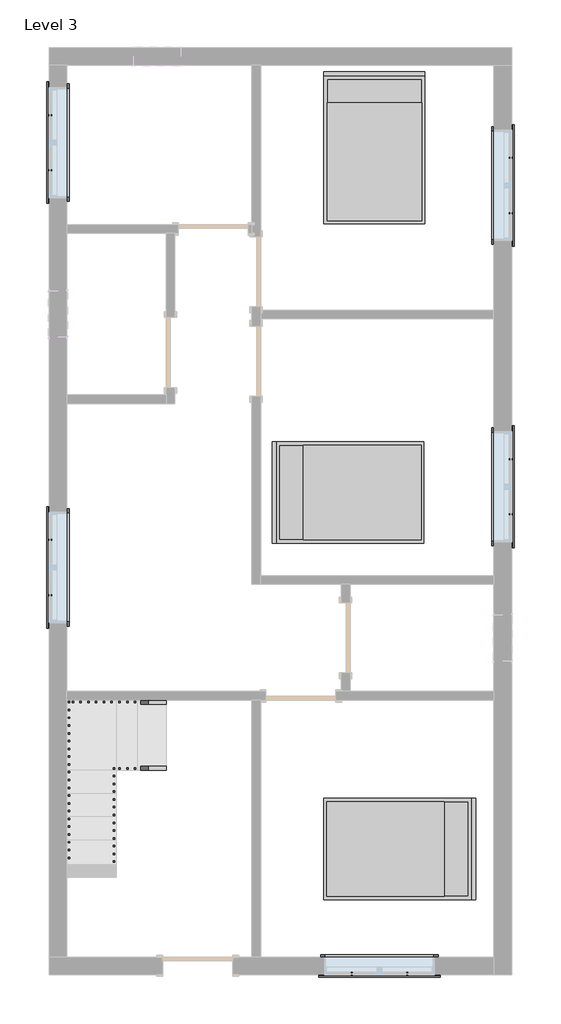
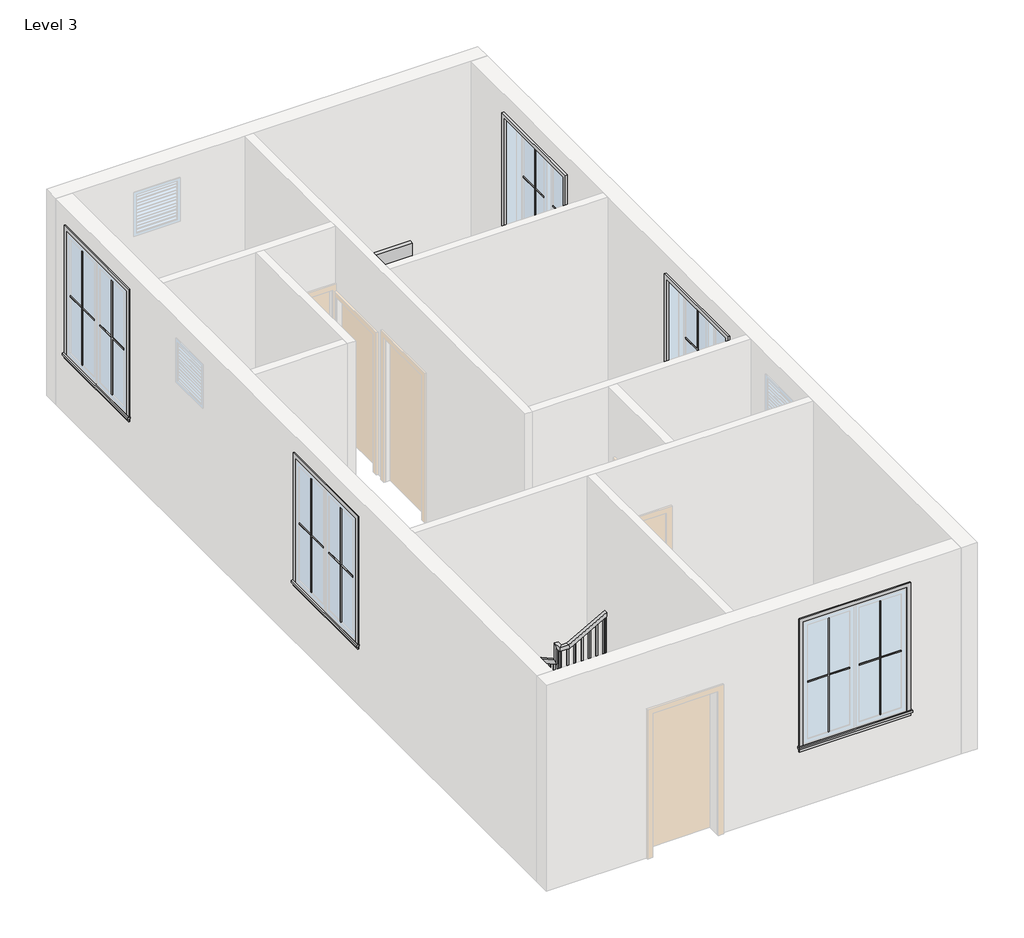
# One storey, part 2 of 2: 20 proxies, 3 furniture elements, 2 railings.
"""IFC4 building model written with IfcOpenShell, lengths in millimetres."""

from ifc_helpers import new_model, si_unit, frame, origin, place, context, project, spatial, polyline, outline, extrude, faceted_brep, transform, mapped, element, save
from components import muntin_pattern_2x2_muntin_pattern_2x2_bff912c5, muntin_pattern_2x2_muntin_pattern_2x2_c2194282, trim_window_exterior_flat_with_sill_e04b3088, trim_window_interior_flat_picture_frame_2a7685fe, bed_17739_bed_17739_15c61121

model = new_model("IFC4")

# Units and contexts
model_context = context("Model", 3, world=origin())
ifc_project = project(units=[si_unit("LENGTHUNIT", "METRE", prefix="MILLI")], contexts=[model_context])

# Site, building, storey
site = spatial("IfcSite", under=ifc_project)
building = spatial("IfcBuilding", under=site)
storey = spatial("IfcBuildingStorey", under=building, Name="Level 3", Elevation=3200.4)

# Proxies
placement = place(None, origin())
muntin_pattern_2x2_muntin_pattern_2x2_shape = muntin_pattern_2x2_muntin_pattern_2x2_bff912c5(model_context)
element("IfcBuildingElementProxy", 1, Name="Muntin Pattern_2x2 : Muntin Pattern_2x2", ObjectType="Muntin Pattern_2x2 : Muntin Pattern_2x2", at=placement, inside=storey, context=model_context, shape_type="MappedRepresentation", body=[
    mapped(muntin_pattern_2x2_muntin_pattern_2x2_shape, transform((-4261.9639285, 4584.2694249, 4184.65), x_axis=(0.0, 1.0, 0.0), y_axis=(-1.0, 0.0, 0.0), z_axis=(0.0, 0.0, 1.0))),
])
element("IfcBuildingElementProxy", 2, Name="Muntin Pattern_2x2 : Muntin Pattern_2x2", ObjectType="Muntin Pattern_2x2 : Muntin Pattern_2x2", at=placement, inside=storey, context=model_context, shape_type="MappedRepresentation", body=[
    mapped(muntin_pattern_2x2_muntin_pattern_2x2_shape, transform((1751.4860715, 4746.1944249, 4184.65), x_axis=(0.0, -1.0, 0.0), y_axis=(1.0, 0.0, 0.0), z_axis=(0.0, 0.0, 1.0))),
])
element("IfcBuildingElementProxy", 3, Name="Muntin Pattern_2x2 : Muntin Pattern_2x2", ObjectType="Muntin Pattern_2x2 : Muntin Pattern_2x2", at=placement, inside=storey, context=model_context, shape_type="MappedRepresentation", body=[
    mapped(muntin_pattern_2x2_muntin_pattern_2x2_shape, transform((-4261.9639285, -962.4555751, 4184.65), x_axis=(0.0, 1.0, 0.0), y_axis=(-1.0, 0.0, 0.0), z_axis=(0.0, 0.0, 1.0))),
])
element("IfcBuildingElementProxy", 4, Name="Muntin Pattern_2x2 : Muntin Pattern_2x2", ObjectType="Muntin Pattern_2x2 : Muntin Pattern_2x2", at=placement, inside=storey, context=model_context, shape_type="MappedRepresentation", body=[
    mapped(muntin_pattern_2x2_muntin_pattern_2x2_shape, transform((1751.4860715, 812.3694249, 4184.65), x_axis=(0.0, -1.0, 0.0), y_axis=(1.0, 0.0, 0.0), z_axis=(0.0, 0.0, 1.0))),
])
element("IfcBuildingElementProxy", 5, Name="Muntin Pattern_2x2 : Muntin Pattern_2x2", ObjectType="Muntin Pattern_2x2 : Muntin Pattern_2x2", at=placement, inside=storey, context=model_context, shape_type="MappedRepresentation", body=[
    mapped(muntin_pattern_2x2_muntin_pattern_2x2_shape, transform((397.3485715, -5907.5180751, 4184.65), x_axis=(-1.0, 0.0, 0.0), y_axis=(0.0, -1.0, 0.0), z_axis=(0.0, 0.0, 1.0))),
])
muntin_pattern_2x2_muntin_pattern_2x2_2_shape = muntin_pattern_2x2_muntin_pattern_2x2_c2194282(model_context)
element("IfcBuildingElementProxy", 6, Name="Muntin Pattern_2x2 : Muntin Pattern_2x2", ObjectType="Muntin Pattern_2x2 : Muntin Pattern_2x2", at=placement, inside=storey, context=model_context, shape_type="MappedRepresentation", body=[
    mapped(muntin_pattern_2x2_muntin_pattern_2x2_2_shape, transform((-4261.9639285, 5304.9944249, 4184.65), x_axis=(0.0, -1.0, 0.0), y_axis=(1.0, 0.0, 0.0), z_axis=(0.0, 0.0, 1.0))),
])
element("IfcBuildingElementProxy", 7, Name="Muntin Pattern_2x2 : Muntin Pattern_2x2", ObjectType="Muntin Pattern_2x2 : Muntin Pattern_2x2", at=placement, inside=storey, context=model_context, shape_type="MappedRepresentation", body=[
    mapped(muntin_pattern_2x2_muntin_pattern_2x2_2_shape, transform((1751.4860715, 4025.4694249, 4184.65), x_axis=(0.0, 1.0, 0.0), y_axis=(-1.0, 0.0, 0.0), z_axis=(0.0, 0.0, 1.0))),
])
element("IfcBuildingElementProxy", 8, Name="Muntin Pattern_2x2 : Muntin Pattern_2x2", ObjectType="Muntin Pattern_2x2 : Muntin Pattern_2x2", at=placement, inside=storey, context=model_context, shape_type="MappedRepresentation", body=[
    mapped(muntin_pattern_2x2_muntin_pattern_2x2_2_shape, transform((-4261.9639285, -241.7305751, 4184.65), x_axis=(0.0, -1.0, 0.0), y_axis=(1.0, 0.0, 0.0), z_axis=(0.0, 0.0, 1.0))),
])
element("IfcBuildingElementProxy", 9, Name="Muntin Pattern_2x2 : Muntin Pattern_2x2", ObjectType="Muntin Pattern_2x2 : Muntin Pattern_2x2", at=placement, inside=storey, context=model_context, shape_type="MappedRepresentation", body=[
    mapped(muntin_pattern_2x2_muntin_pattern_2x2_2_shape, transform((1751.4860715, 91.6444249, 4184.65), x_axis=(0.0, 1.0, 0.0), y_axis=(-1.0, 0.0, 0.0), z_axis=(0.0, 0.0, 1.0))),
])
element("IfcBuildingElementProxy", 10, Name="Muntin Pattern_2x2 : Muntin Pattern_2x2", ObjectType="Muntin Pattern_2x2 : Muntin Pattern_2x2", at=placement, inside=storey, context=model_context, shape_type="MappedRepresentation", body=[
    mapped(muntin_pattern_2x2_muntin_pattern_2x2_2_shape, transform((-323.3764285, -5907.5180751, 4184.65), x_axis=(1.0, 0.0, 0.0), y_axis=(0.0, 1.0, 0.0), z_axis=(0.0, 0.0, 1.0))),
])
trim_window_exterior_flat_with_sill_shape = trim_window_exterior_flat_with_sill_e04b3088(model_context)
element("IfcBuildingElementProxy", 11, Name="Trim-Window-Exterior-Flat : with Sill", ObjectType="Trim-Window-Exterior-Flat : with Sill", at=placement, inside=storey, context=model_context, shape_type="MappedRepresentation", body=[
    mapped(trim_window_exterior_flat_with_sill_shape, transform((-4271.4889285, 4944.6319249, 5943.6), x_axis=(0.0, -1.0, 0.0), y_axis=(0.0, 0.0, 1.0), z_axis=(-1.0, 0.0, 0.0))),
])
element("IfcBuildingElementProxy", 12, Name="Trim-Window-Exterior-Flat : with Sill", ObjectType="Trim-Window-Exterior-Flat : with Sill", at=placement, inside=storey, context=model_context, shape_type="MappedRepresentation", body=[
    mapped(trim_window_exterior_flat_with_sill_shape, transform((1761.0110715, 4385.8319249, 5943.6), x_axis=(0.0, 1.0, 0.0), y_axis=(0.0, 0.0, 1.0), z_axis=(1.0, 0.0, 0.0))),
])
element("IfcBuildingElementProxy", 13, Name="Trim-Window-Exterior-Flat : with Sill", ObjectType="Trim-Window-Exterior-Flat : with Sill", at=placement, inside=storey, context=model_context, shape_type="MappedRepresentation", body=[
    mapped(trim_window_exterior_flat_with_sill_shape, transform((-4271.4889285, -602.0930751, 5943.6), x_axis=(0.0, -1.0, 0.0), y_axis=(0.0, 0.0, 1.0), z_axis=(-1.0, 0.0, 0.0))),
])
element("IfcBuildingElementProxy", 14, Name="Trim-Window-Exterior-Flat : with Sill", ObjectType="Trim-Window-Exterior-Flat : with Sill", at=placement, inside=storey, context=model_context, shape_type="MappedRepresentation", body=[
    mapped(trim_window_exterior_flat_with_sill_shape, transform((1761.0110715, 452.0069249, 5943.6), x_axis=(0.0, 1.0, 0.0), y_axis=(0.0, 0.0, 1.0), z_axis=(1.0, 0.0, 0.0))),
])
element("IfcBuildingElementProxy", 15, Name="Trim-Window-Exterior-Flat : with Sill", ObjectType="Trim-Window-Exterior-Flat : with Sill", at=placement, inside=storey, context=model_context, shape_type="MappedRepresentation", body=[
    mapped(trim_window_exterior_flat_with_sill_shape, transform((36.9860715, -5917.0430751, 5943.6), x_axis=(1.0, 0.0, 0.0), y_axis=(0.0, 0.0, 1.0), z_axis=(0.0, -1.0, 0.0))),
])
trim_window_interior_flat_picture_frame_shape = trim_window_interior_flat_picture_frame_2a7685fe(model_context)
element("IfcBuildingElementProxy", 16, Name="Trim-Window-Interior-Flat : Picture Frame", ObjectType="Trim-Window-Interior-Flat : Picture Frame", at=placement, inside=storey, context=model_context, shape_type="MappedRepresentation", body=[
    mapped(trim_window_interior_flat_picture_frame_shape, transform((-4042.8889285, 4944.6319249, 5943.6), x_axis=(0.0, 1.0, 0.0), y_axis=(0.0, 0.0, 1.0), z_axis=(1.0, 0.0, 0.0))),
])
element("IfcBuildingElementProxy", 17, Name="Trim-Window-Interior-Flat : Picture Frame", ObjectType="Trim-Window-Interior-Flat : Picture Frame", at=placement, inside=storey, context=model_context, shape_type="MappedRepresentation", body=[
    mapped(trim_window_interior_flat_picture_frame_shape, transform((1532.4110715, 4385.8319249, 5943.6), x_axis=(0.0, -1.0, 0.0), y_axis=(0.0, 0.0, 1.0), z_axis=(-1.0, 0.0, 0.0))),
])
element("IfcBuildingElementProxy", 18, Name="Trim-Window-Interior-Flat : Picture Frame", ObjectType="Trim-Window-Interior-Flat : Picture Frame", at=placement, inside=storey, context=model_context, shape_type="MappedRepresentation", body=[
    mapped(trim_window_interior_flat_picture_frame_shape, transform((-4042.8889285, -602.0930751, 5943.6), x_axis=(0.0, 1.0, 0.0), y_axis=(0.0, 0.0, 1.0), z_axis=(1.0, 0.0, 0.0))),
])
element("IfcBuildingElementProxy", 19, Name="Trim-Window-Interior-Flat : Picture Frame", ObjectType="Trim-Window-Interior-Flat : Picture Frame", at=placement, inside=storey, context=model_context, shape_type="MappedRepresentation", body=[
    mapped(trim_window_interior_flat_picture_frame_shape, transform((1532.4110715, 452.0069249, 5943.6), x_axis=(0.0, -1.0, 0.0), y_axis=(0.0, 0.0, 1.0), z_axis=(-1.0, 0.0, 0.0))),
])
element("IfcBuildingElementProxy", 20, Name="Trim-Window-Interior-Flat : Picture Frame", ObjectType="Trim-Window-Interior-Flat : Picture Frame", at=placement, inside=storey, context=model_context, shape_type="MappedRepresentation", body=[
    mapped(trim_window_interior_flat_picture_frame_shape, transform((36.9860715, -5688.4430751, 5943.6), x_axis=(-1.0, 0.0, 0.0), y_axis=(0.0, 0.0, 1.0), z_axis=(0.0, 1.0, 0.0))),
])

# Furniture
bed_17739_bed_17739_shape = bed_17739_bed_17739_15c61121(model_context)
element("IfcFurniture", 21, ObjectType="Bed_17739 : Bed_17739", at=placement, inside=storey, context=model_context, shape_type="MappedRepresentation", body=[
    mapped(bed_17739_bed_17739_shape, transform((-29.6889285, 4852.5569249, 3200.4), x_axis=(1.0, 0.0, 0.0), y_axis=(0.0, 1.0, 0.0), z_axis=(0.0, 0.0, 1.0))),
])
element("IfcFurniture", 22, ObjectType="Bed_17739 : Bed_17739", at=placement, inside=storey, context=model_context, shape_type="MappedRepresentation", body=[
    mapped(bed_17739_bed_17739_shape, transform((-347.1889285, 375.8069249, 3200.4), x_axis=(0.0, 1.0, 0.0), y_axis=(-1.0, 0.0, 0.0), z_axis=(0.0, 0.0, 1.0))),
])
element("IfcFurniture", 23, ObjectType="Bed_17739 : Bed_17739", at=placement, inside=storey, context=model_context, shape_type="MappedRepresentation", body=[
    mapped(bed_17739_bed_17739_shape, transform((275.1110715, -4278.7430751, 3200.4), x_axis=(0.0, -1.0, 0.0), y_axis=(1.0, 0.0, 0.0), z_axis=(0.0, 0.0, 1.0))),
])

# Railings
element("IfcRailing", 24, ObjectType="Handrail - Rectangular", at=placement, inside=storey, context=model_context, shape_type="SolidModel", body=[
    faceted_brep([(-2747.4889285, -2386.4430751, 4284.1333333), (-2747.4889285, -2386.4430751, 4226.9271159), (-2747.4889285, -2335.6430751, 4226.9271159), (-2747.4889285, -2335.6430751, 4284.1333333), (-3396.0267484, -2386.4430751, 4619.9457967), (-3408.3987558, -2386.4430751, 4569.1457967), (-3408.3987558, -2335.6430751, 4569.1457967), (-3396.0267484, -2335.6430751, 4619.9457967), (-3992.0889285, -2386.4430751, 4619.9457967), (-3992.0889285, -2386.4430751, 4569.1457967), (-4042.8889285, -2335.6430751, 4569.1457967), (-4042.8889285, -2335.6430751, 4619.9457967), (-3992.0889285, -2940.1628326, 4619.9457967), (-3992.0889285, -2953.3285634, 4569.1457967), (-4042.8889285, -2953.3285634, 4569.1457967), (-4042.8889285, -2940.1628326, 4619.9457967), (-3992.0889285, -5061.9991591, 5798.9618165), (-3992.0889285, -5075.1648899, 5748.1618165), (-4042.8889285, -5075.1648899, 5748.1618165), (-4042.8889285, -5061.9991591, 5798.9618165), (-3992.0889285, -5637.6430751, 5798.9618165), (-3992.0889285, -5637.6430751, 5748.1618165), (-4042.8889285, -5688.4430751, 5748.1618165), (-4042.8889285, -5688.4430751, 5798.9618165), (-3418.001852, -5637.6430751, 5798.9618165), (-3404.8062484, -5637.6430751, 5748.1618165), (-3404.8062484, -5688.4430751, 5748.1618165), (-3418.001852, -5688.4430751, 5798.9618165), (-2793.6303845, -5637.6430751, 6146.8), (-2793.6303845, -5688.4430751, 6146.8), (-2793.6303845, -5688.4430751, 6088.6487115), (-2793.6303845, -5637.6430751, 6088.6487115)], [[[0, 1, 2, 3]], [[1, 0, 4, 5]], [[2, 1, 5, 6]], [[3, 2, 6, 7]], [[0, 3, 7, 4]], [[5, 4, 8, 9]], [[6, 5, 9, 10]], [[7, 6, 10, 11]], [[4, 7, 11, 8]], [[9, 8, 12, 13]], [[10, 9, 13, 14]], [[11, 10, 14, 15]], [[8, 11, 15, 12]], [[13, 12, 16, 17]], [[14, 13, 17, 18]], [[15, 14, 18, 19]], [[12, 15, 19, 16]], [[17, 16, 20, 21]], [[18, 17, 21, 22]], [[19, 18, 22, 23]], [[16, 19, 23, 20]], [[21, 20, 24, 25]], [[22, 21, 25, 26]], [[23, 22, 26, 27]], [[20, 23, 27, 24]], [[28, 29, 30, 31]], [[25, 24, 28, 31]], [[26, 25, 31, 30]], [[27, 26, 30, 29]], [[24, 27, 29, 28]]]),
    extrude(outline(polyline([(6091.3598207, -2788.7639285), (6080.7470401, -2807.8139285), (5063.0666667, -2807.8139285), (5063.0666667, -2788.7639285), (6091.3598207, -2788.7639285)])), frame((0.0, -5672.5680751, 0.0), z_axis=(0.0, 1.0, 0.0), x_axis=(0.0, 0.0, 1.0)), (0.0, 0.0, 1.0), 19.05),
    extrude(outline(polyline([(6034.7583242, -2890.3639285), (6024.1455436, -2909.4139285), (5063.0666667, -2909.4139285), (5063.0666667, -2890.3639285), (6034.7583242, -2890.3639285)])), frame((0.0, -5672.5680751, 0.0), z_axis=(0.0, 1.0, 0.0), x_axis=(0.0, 0.0, 1.0)), (0.0, 0.0, 1.0), 19.05),
    extrude(outline(polyline([(5978.1568277, -2991.9639285), (5967.5440471, -3011.0139285), (5063.0666667, -3011.0139285), (5063.0666667, -2991.9639285), (5978.1568277, -2991.9639285)])), frame((0.0, -5672.5680751, 0.0), z_axis=(0.0, 1.0, 0.0), x_axis=(0.0, 0.0, 1.0)), (0.0, 0.0, 1.0), 19.05),
    extrude(outline(polyline([(5921.5553312, -3093.5639285), (5910.9425506, -3112.6139285), (5063.0666667, -3112.6139285), (5063.0666667, -3093.5639285), (5921.5553312, -3093.5639285)])), frame((0.0, -5672.5680751, 0.0), z_axis=(0.0, 1.0, 0.0), x_axis=(0.0, 0.0, 1.0)), (0.0, 0.0, 1.0), 19.05),
    extrude(outline(polyline([(5864.9538346, -3195.1639285), (5854.3410541, -3214.2139285), (4893.7333333, -3214.2139285), (4893.7333333, -3195.1639285), (5864.9538346, -3195.1639285)])), frame((0.0, -5672.5680751, 0.0), z_axis=(0.0, 1.0, 0.0), x_axis=(0.0, 0.0, 1.0)), (0.0, 0.0, 1.0), 19.05),
    extrude(outline(polyline([(5808.3523381, -3296.7639285), (5797.7395575, -3315.8139285), (4893.7333333, -3315.8139285), (4893.7333333, -3296.7639285), (5808.3523381, -3296.7639285)])), frame((0.0, -5672.5680751, 0.0), z_axis=(0.0, 1.0, 0.0), x_axis=(0.0, 0.0, 1.0)), (0.0, 0.0, 1.0), 19.05),
    extrude(outline(polyline([(5751.7508416, -3398.3639285), (5741.138061, -3417.4139285), (4724.4, -3417.4139285), (4724.4, -3398.3639285), (5751.7508416, -3398.3639285)])), frame((0.0, -5672.5680751, 0.0), z_axis=(0.0, 1.0, 0.0), x_axis=(0.0, 0.0, 1.0)), (0.0, 0.0, 1.0), 19.05),
    extrude(outline(polyline([(-3519.0139285, -5672.5680751), (-3519.0139285, -5653.5180751), (-3499.9639285, -5653.5180751), (-3499.9639285, -5672.5680751), (-3519.0139285, -5672.5680751)])), frame((0.0, 0.0, 4724.4), z_axis=(0.0, 0.0, 1.0), x_axis=(1.0, 0.0, 0.0)), (0.0, 0.0, 1.0), 1023.7618165),
    extrude(outline(polyline([(-3620.6139285, -5672.5680751), (-3620.6139285, -5653.5180751), (-3601.5639285, -5653.5180751), (-3601.5639285, -5672.5680751), (-3620.6139285, -5672.5680751)])), frame((0.0, 0.0, 4724.4), z_axis=(0.0, 0.0, 1.0), x_axis=(1.0, 0.0, 0.0)), (0.0, 0.0, 1.0), 1023.7618165),
    extrude(outline(polyline([(-3722.2139285, -5672.5680751), (-3722.2139285, -5653.5180751), (-3703.1639285, -5653.5180751), (-3703.1639285, -5672.5680751), (-3722.2139285, -5672.5680751)])), frame((0.0, 0.0, 4724.4), z_axis=(0.0, 0.0, 1.0), x_axis=(1.0, 0.0, 0.0)), (0.0, 0.0, 1.0), 1023.7618165),
    extrude(outline(polyline([(-3823.8139285, -5672.5680751), (-3823.8139285, -5653.5180751), (-3804.7639285, -5653.5180751), (-3804.7639285, -5672.5680751), (-3823.8139285, -5672.5680751)])), frame((0.0, 0.0, 4724.4), z_axis=(0.0, 0.0, 1.0), x_axis=(1.0, 0.0, 0.0)), (0.0, 0.0, 1.0), 1023.7618165),
    extrude(outline(polyline([(-3925.4139285, -5672.5680751), (-3925.4139285, -5653.5180751), (-3906.3639285, -5653.5180751), (-3906.3639285, -5672.5680751), (-3925.4139285, -5672.5680751)])), frame((0.0, 0.0, 4724.4), z_axis=(0.0, 0.0, 1.0), x_axis=(1.0, 0.0, 0.0)), (0.0, 0.0, 1.0), 1023.7618165),
    extrude(outline(polyline([(-4027.0139285, -5602.7180751), (-4007.9639285, -5602.7180751), (-4007.9639285, -5621.7680751), (-4027.0139285, -5621.7680751), (-4027.0139285, -5602.7180751)])), frame((0.0, 0.0, 4724.4), z_axis=(0.0, 0.0, 1.0), x_axis=(1.0, 0.0, 0.0)), (0.0, 0.0, 1.0), 1023.7618165),
    extrude(outline(polyline([(-4027.0139285, -5501.1180751), (-4007.9639285, -5501.1180751), (-4007.9639285, -5520.1680751), (-4027.0139285, -5520.1680751), (-4027.0139285, -5501.1180751)])), frame((0.0, 0.0, 4724.4), z_axis=(0.0, 0.0, 1.0), x_axis=(1.0, 0.0, 0.0)), (0.0, 0.0, 1.0), 1023.7618165),
    extrude(outline(polyline([(-4027.0139285, -5399.5180751), (-4007.9639285, -5399.5180751), (-4007.9639285, -5418.5680751), (-4027.0139285, -5418.5680751), (-4027.0139285, -5399.5180751)])), frame((0.0, 0.0, 4724.4), z_axis=(0.0, 0.0, 1.0), x_axis=(1.0, 0.0, 0.0)), (0.0, 0.0, 1.0), 1023.7618165),
    extrude(outline(polyline([(-4027.0139285, -5297.9180751), (-4007.9639285, -5297.9180751), (-4007.9639285, -5316.9680751), (-4027.0139285, -5316.9680751), (-4027.0139285, -5297.9180751)])), frame((0.0, 0.0, 4724.4), z_axis=(0.0, 0.0, 1.0), x_axis=(1.0, 0.0, 0.0)), (0.0, 0.0, 1.0), 1023.7618165),
    extrude(outline(polyline([(-4027.0139285, -5196.3180751), (-4007.9639285, -5196.3180751), (-4007.9639285, -5215.3680751), (-4027.0139285, -5215.3680751), (-4027.0139285, -5196.3180751)])), frame((0.0, 0.0, 4724.4), z_axis=(0.0, 0.0, 1.0), x_axis=(1.0, 0.0, 0.0)), (0.0, 0.0, 1.0), 1023.7618165),
    extrude(outline(polyline([(-4027.0139285, -5094.7180751), (-4007.9639285, -5094.7180751), (-4007.9639285, -5113.7680751), (-4027.0139285, -5113.7680751), (-4027.0139285, -5094.7180751)])), frame((0.0, 0.0, 4724.4), z_axis=(0.0, 0.0, 1.0), x_axis=(1.0, 0.0, 0.0)), (0.0, 0.0, 1.0), 1023.7618165),
    extrude(outline(polyline([(-5012.1680751, 5713.1571119), (-4993.1180751, 5702.5718208), (-4993.1180751, 4724.4), (-5012.1680751, 4724.4), (-5012.1680751, 5713.1571119)])), frame((-4027.0139285, 0.0, 0.0), z_axis=(1.0, 0.0, 0.0), x_axis=(0.0, 1.0, 0.0)), (0.0, 0.0, 1.0), 19.05),
    extrude(outline(polyline([(-4910.5680751, 5656.7022261), (-4891.5180751, 5646.116935), (-4891.5180751, 4724.4), (-4910.5680751, 4724.4), (-4910.5680751, 5656.7022261)])), frame((-4027.0139285, 0.0, 0.0), z_axis=(1.0, 0.0, 0.0), x_axis=(0.0, 1.0, 0.0)), (0.0, 0.0, 1.0), 19.05),
    extrude(outline(polyline([(-4808.9680751, 5600.2473402), (-4789.9180751, 5589.6620491), (-4789.9180751, 4724.4), (-4808.9680751, 4724.4), (-4808.9680751, 5600.2473402)])), frame((-4027.0139285, 0.0, 0.0), z_axis=(1.0, 0.0, 0.0), x_axis=(0.0, 1.0, 0.0)), (0.0, 0.0, 1.0), 19.05),
    extrude(outline(polyline([(-4707.3680751, 5543.6358332), (-4688.3180751, 5533.0505421), (-4688.3180751, 4555.0666667), (-4707.3680751, 4555.0666667), (-4707.3680751, 5543.6358332)])), frame((-4027.0139285, 0.0, 0.0), z_axis=(1.0, 0.0, 0.0), x_axis=(0.0, 1.0, 0.0)), (0.0, 0.0, 1.0), 19.05),
    extrude(outline(polyline([(-4605.7680751, 5487.1809474), (-4586.7180751, 5476.5956563), (-4586.7180751, 4555.0666667), (-4605.7680751, 4555.0666667), (-4605.7680751, 5487.1809474)])), frame((-4027.0139285, 0.0, 0.0), z_axis=(1.0, 0.0, 0.0), x_axis=(0.0, 1.0, 0.0)), (0.0, 0.0, 1.0), 19.05),
    extrude(outline(polyline([(-4504.1680751, 5430.7260615), (-4485.1180751, 5420.1407704), (-4485.1180751, 4555.0666667), (-4504.1680751, 4555.0666667), (-4504.1680751, 5430.7260615)])), frame((-4027.0139285, 0.0, 0.0), z_axis=(1.0, 0.0, 0.0), x_axis=(0.0, 1.0, 0.0)), (0.0, 0.0, 1.0), 19.05),
    extrude(outline(polyline([(-4402.5680751, 5374.3024999), (-4383.5180751, 5363.7172088), (-4383.5180751, 4385.7333333), (-4402.5680751, 4385.7333333), (-4402.5680751, 5374.3024999)])), frame((-4027.0139285, 0.0, 0.0), z_axis=(1.0, 0.0, 0.0), x_axis=(0.0, 1.0, 0.0)), (0.0, 0.0, 1.0), 19.05),
    extrude(outline(polyline([(-4300.9680751, 5317.847614), (-4281.9180751, 5307.2623229), (-4281.9180751, 4385.7333333), (-4300.9680751, 4385.7333333), (-4300.9680751, 5317.847614)])), frame((-4027.0139285, 0.0, 0.0), z_axis=(1.0, 0.0, 0.0), x_axis=(0.0, 1.0, 0.0)), (0.0, 0.0, 1.0), 19.05),
    extrude(outline(polyline([(-4199.3680751, 5261.3927282), (-4180.3180751, 5250.8074371), (-4180.3180751, 4385.7333333), (-4199.3680751, 4385.7333333), (-4199.3680751, 5261.3927282)])), frame((-4027.0139285, 0.0, 0.0), z_axis=(1.0, 0.0, 0.0), x_axis=(0.0, 1.0, 0.0)), (0.0, 0.0, 1.0), 19.05),
    extrude(outline(polyline([(-4097.7680751, 5204.9691666), (-4078.7180751, 5194.3838755), (-4078.7180751, 4216.4), (-4097.7680751, 4216.4), (-4097.7680751, 5204.9691666)])), frame((-4027.0139285, 0.0, 0.0), z_axis=(1.0, 0.0, 0.0), x_axis=(0.0, 1.0, 0.0)), (0.0, 0.0, 1.0), 19.05),
    extrude(outline(polyline([(-3996.1680751, 5148.5142807), (-3977.1180751, 5137.9289896), (-3977.1180751, 4216.4), (-3996.1680751, 4216.4), (-3996.1680751, 5148.5142807)])), frame((-4027.0139285, 0.0, 0.0), z_axis=(1.0, 0.0, 0.0), x_axis=(0.0, 1.0, 0.0)), (0.0, 0.0, 1.0), 19.05),
    extrude(outline(polyline([(-3894.5680751, 5092.0593949), (-3875.5180751, 5081.4741038), (-3875.5180751, 4216.4), (-3894.5680751, 4216.4), (-3894.5680751, 5092.0593949)])), frame((-4027.0139285, 0.0, 0.0), z_axis=(1.0, 0.0, 0.0), x_axis=(0.0, 1.0, 0.0)), (0.0, 0.0, 1.0), 19.05),
    extrude(outline(polyline([(-3792.9680751, 5035.6358332), (-3773.9180751, 5025.0505421), (-3773.9180751, 4047.0666667), (-3792.9680751, 4047.0666667), (-3792.9680751, 5035.6358332)])), frame((-4027.0139285, 0.0, 0.0), z_axis=(1.0, 0.0, 0.0), x_axis=(0.0, 1.0, 0.0)), (0.0, 0.0, 1.0), 19.05),
    extrude(outline(polyline([(-3691.3680751, 4979.1809474), (-3672.3180751, 4968.5956563), (-3672.3180751, 4047.0666667), (-3691.3680751, 4047.0666667), (-3691.3680751, 4979.1809474)])), frame((-4027.0139285, 0.0, 0.0), z_axis=(1.0, 0.0, 0.0), x_axis=(0.0, 1.0, 0.0)), (0.0, 0.0, 1.0), 19.05),
    extrude(outline(polyline([(-3589.7680751, 4922.7260615), (-3570.7180751, 4912.1407704), (-3570.7180751, 4047.0666667), (-3589.7680751, 4047.0666667), (-3589.7680751, 4922.7260615)])), frame((-4027.0139285, 0.0, 0.0), z_axis=(1.0, 0.0, 0.0), x_axis=(0.0, 1.0, 0.0)), (0.0, 0.0, 1.0), 19.05),
    extrude(outline(polyline([(-3488.1680751, 4866.3024999), (-3469.1180751, 4855.7172088), (-3469.1180751, 3877.7333333), (-3488.1680751, 3877.7333333), (-3488.1680751, 4866.3024999)])), frame((-4027.0139285, 0.0, 0.0), z_axis=(1.0, 0.0, 0.0), x_axis=(0.0, 1.0, 0.0)), (0.0, 0.0, 1.0), 19.05),
    extrude(outline(polyline([(-3386.5680751, 4809.847614), (-3367.5180751, 4799.2623229), (-3367.5180751, 3877.7333333), (-3386.5680751, 3877.7333333), (-3386.5680751, 4809.847614)])), frame((-4027.0139285, 0.0, 0.0), z_axis=(1.0, 0.0, 0.0), x_axis=(0.0, 1.0, 0.0)), (0.0, 0.0, 1.0), 19.05),
    extrude(outline(polyline([(-3284.9680751, 4753.3927282), (-3265.9180751, 4742.8074371), (-3265.9180751, 3877.7333333), (-3284.9680751, 3877.7333333), (-3284.9680751, 4753.3927282)])), frame((-4027.0139285, 0.0, 0.0), z_axis=(1.0, 0.0, 0.0), x_axis=(0.0, 1.0, 0.0)), (0.0, 0.0, 1.0), 19.05),
    extrude(outline(polyline([(-3183.3680751, 4696.9691666), (-3164.3180751, 4686.3838755), (-3164.3180751, 3708.4), (-3183.3680751, 3708.4), (-3183.3680751, 4696.9691666)])), frame((-4027.0139285, 0.0, 0.0), z_axis=(1.0, 0.0, 0.0), x_axis=(0.0, 1.0, 0.0)), (0.0, 0.0, 1.0), 19.05),
    extrude(outline(polyline([(-3081.7680751, 4640.5142807), (-3062.7180751, 4629.9289896), (-3062.7180751, 3708.4), (-3081.7680751, 3708.4), (-3081.7680751, 4640.5142807)])), frame((-4027.0139285, 0.0, 0.0), z_axis=(1.0, 0.0, 0.0), x_axis=(0.0, 1.0, 0.0)), (0.0, 0.0, 1.0), 19.05),
    extrude(outline(polyline([(-2980.1680751, 4584.0593949), (-2961.1180751, 4573.4741038), (-2961.1180751, 3708.4), (-2980.1680751, 3708.4), (-2980.1680751, 4584.0593949)])), frame((-4027.0139285, 0.0, 0.0), z_axis=(1.0, 0.0, 0.0), x_axis=(0.0, 1.0, 0.0)), (0.0, 0.0, 1.0), 19.05),
    extrude(outline(polyline([(-4027.0139285, -2859.5180751), (-4007.9639285, -2859.5180751), (-4007.9639285, -2878.5680751), (-4027.0139285, -2878.5680751), (-4027.0139285, -2859.5180751)])), frame((0.0, 0.0, 3708.4), z_axis=(0.0, 0.0, 1.0), x_axis=(1.0, 0.0, 0.0)), (0.0, 0.0, 1.0), 860.7457967),
    extrude(outline(polyline([(-4027.0139285, -2757.9180751), (-4007.9639285, -2757.9180751), (-4007.9639285, -2776.9680751), (-4027.0139285, -2776.9680751), (-4027.0139285, -2757.9180751)])), frame((0.0, 0.0, 3708.4), z_axis=(0.0, 0.0, 1.0), x_axis=(1.0, 0.0, 0.0)), (0.0, 0.0, 1.0), 860.7457967),
    extrude(outline(polyline([(-4027.0139285, -2656.3180751), (-4007.9639285, -2656.3180751), (-4007.9639285, -2675.3680751), (-4027.0139285, -2675.3680751), (-4027.0139285, -2656.3180751)])), frame((0.0, 0.0, 3708.4), z_axis=(0.0, 0.0, 1.0), x_axis=(1.0, 0.0, 0.0)), (0.0, 0.0, 1.0), 860.7457967),
    extrude(outline(polyline([(-4027.0139285, -2554.7180751), (-4007.9639285, -2554.7180751), (-4007.9639285, -2573.7680751), (-4027.0139285, -2573.7680751), (-4027.0139285, -2554.7180751)])), frame((0.0, 0.0, 3708.4), z_axis=(0.0, 0.0, 1.0), x_axis=(1.0, 0.0, 0.0)), (0.0, 0.0, 1.0), 860.7457967),
    extrude(outline(polyline([(-4027.0139285, -2453.1180751), (-4007.9639285, -2453.1180751), (-4007.9639285, -2472.1680751), (-4027.0139285, -2472.1680751), (-4027.0139285, -2453.1180751)])), frame((0.0, 0.0, 3708.4), z_axis=(0.0, 0.0, 1.0), x_axis=(1.0, 0.0, 0.0)), (0.0, 0.0, 1.0), 860.7457967),
    extrude(outline(polyline([(-3957.1639285, -2351.5180751), (-3957.1639285, -2370.5680751), (-3976.2139285, -2370.5680751), (-3976.2139285, -2351.5180751), (-3957.1639285, -2351.5180751)])), frame((0.0, 0.0, 3708.4), z_axis=(0.0, 0.0, 1.0), x_axis=(1.0, 0.0, 0.0)), (0.0, 0.0, 1.0), 860.7457967),
    extrude(outline(polyline([(-3855.5639285, -2351.5180751), (-3855.5639285, -2370.5680751), (-3874.6139285, -2370.5680751), (-3874.6139285, -2351.5180751), (-3855.5639285, -2351.5180751)])), frame((0.0, 0.0, 3708.4), z_axis=(0.0, 0.0, 1.0), x_axis=(1.0, 0.0, 0.0)), (0.0, 0.0, 1.0), 860.7457967),
    extrude(outline(polyline([(-3753.9639285, -2351.5180751), (-3753.9639285, -2370.5680751), (-3773.0139285, -2370.5680751), (-3773.0139285, -2351.5180751), (-3753.9639285, -2351.5180751)])), frame((0.0, 0.0, 3708.4), z_axis=(0.0, 0.0, 1.0), x_axis=(1.0, 0.0, 0.0)), (0.0, 0.0, 1.0), 860.7457967),
    extrude(outline(polyline([(-3652.3639285, -2351.5180751), (-3652.3639285, -2370.5680751), (-3671.4139285, -2370.5680751), (-3671.4139285, -2351.5180751), (-3652.3639285, -2351.5180751)])), frame((0.0, 0.0, 3708.4), z_axis=(0.0, 0.0, 1.0), x_axis=(1.0, 0.0, 0.0)), (0.0, 0.0, 1.0), 860.7457967),
    extrude(outline(polyline([(-3550.7639285, -2351.5180751), (-3550.7639285, -2370.5680751), (-3569.8139285, -2370.5680751), (-3569.8139285, -2351.5180751), (-3550.7639285, -2351.5180751)])), frame((0.0, 0.0, 3708.4), z_axis=(0.0, 0.0, 1.0), x_axis=(1.0, 0.0, 0.0)), (0.0, 0.0, 1.0), 860.7457967),
    extrude(outline(polyline([(-3449.1639285, -2351.5180751), (-3449.1639285, -2370.5680751), (-3468.2139285, -2370.5680751), (-3468.2139285, -2351.5180751), (-3449.1639285, -2351.5180751)])), frame((0.0, 0.0, 3708.4), z_axis=(0.0, 0.0, 1.0), x_axis=(1.0, 0.0, 0.0)), (0.0, 0.0, 1.0), 860.7457967),
    extrude(outline(polyline([(4537.6455625, -3347.5639285), (4547.5096402, -3366.6139285), (3539.0666667, -3366.6139285), (3539.0666667, -3347.5639285), (4537.6455625, -3347.5639285)])), frame((0.0, -2370.5680751, 0.0), z_axis=(0.0, 1.0, 0.0), x_axis=(0.0, 0.0, 1.0)), (0.0, 0.0, 1.0), 19.05),
    extrude(outline(polyline([(4485.0371483, -3245.9639285), (4494.9012259, -3265.0139285), (3539.0666667, -3265.0139285), (3539.0666667, -3245.9639285), (4485.0371483, -3245.9639285)])), frame((0.0, -2370.5680751, 0.0), z_axis=(0.0, 1.0, 0.0), x_axis=(0.0, 0.0, 1.0)), (0.0, 0.0, 1.0), 19.05),
    extrude(outline(polyline([(4432.428734, -3144.3639285), (4442.2928117, -3163.4139285), (3539.0666667, -3163.4139285), (3539.0666667, -3144.3639285), (4432.428734, -3144.3639285)])), frame((0.0, -2370.5680751, 0.0), z_axis=(0.0, 1.0, 0.0), x_axis=(0.0, 0.0, 1.0)), (0.0, 0.0, 1.0), 19.05),
    extrude(outline(polyline([(4379.8203198, -3042.7639285), (4389.6843975, -3061.8139285), (3369.7333333, -3061.8139285), (3369.7333333, -3042.7639285), (4379.8203198, -3042.7639285)])), frame((0.0, -2370.5680751, 0.0), z_axis=(0.0, 1.0, 0.0), x_axis=(0.0, 0.0, 1.0)), (0.0, 0.0, 1.0), 19.05),
    extrude(outline(polyline([(4327.2119056, -2941.1639285), (4337.0759832, -2960.2139285), (3369.7333333, -2960.2139285), (3369.7333333, -2941.1639285), (4327.2119056, -2941.1639285)])), frame((0.0, -2370.5680751, 0.0), z_axis=(0.0, 1.0, 0.0), x_axis=(0.0, 0.0, 1.0)), (0.0, 0.0, 1.0), 19.05),
    extrude(outline(polyline([(4274.6034913, -2839.5639285), (4284.467569, -2858.6139285), (3369.7333333, -2858.6139285), (3369.7333333, -2839.5639285), (4274.6034913, -2839.5639285)])), frame((0.0, -2370.5680751, 0.0), z_axis=(0.0, 1.0, 0.0), x_axis=(0.0, 0.0, 1.0)), (0.0, 0.0, 1.0), 19.05),
    extrude(outline(polyline([(-4027.0139285, -5653.5180751), (-4007.9639285, -5653.5180751), (-4007.9639285, -5672.5680751), (-4027.0139285, -5672.5680751), (-4027.0139285, -5653.5180751)])), frame((0.0, 0.0, 4724.4), z_axis=(0.0, 0.0, 1.0), x_axis=(1.0, 0.0, 0.0)), (0.0, 0.0, 1.0), 1023.7618165),
    extrude(outline(polyline([(-4007.9639285, -2351.5180751), (-4007.9639285, -2370.5680751), (-4027.0139285, -2370.5680751), (-4027.0139285, -2351.5180751), (-4007.9639285, -2351.5180751)])), frame((0.0, 0.0, 3708.4), z_axis=(0.0, 0.0, 1.0), x_axis=(1.0, 0.0, 0.0)), (0.0, 0.0, 1.0), 860.7457967),
    extrude(outline(polyline([(6088.6487115, -2793.6303845), (6078.0359309, -2812.6803845), (5063.0666667, -2812.6803845), (5063.0666667, -2793.6303845), (6088.6487115, -2793.6303845)])), frame((0.0, -5672.5680751, 0.0), z_axis=(0.0, 1.0, 0.0), x_axis=(0.0, 0.0, 1.0)), (0.0, 0.0, 1.0), 19.05),
    extrude(outline(polyline([(4226.9271159, -2747.4889285), (4236.7911936, -2766.5389285), (3369.7333333, -2766.5389285), (3369.7333333, -2747.4889285), (4226.9271159, -2747.4889285)])), frame((0.0, -2370.5680751, 0.0), z_axis=(0.0, 1.0, 0.0), x_axis=(0.0, 0.0, 1.0)), (0.0, 0.0, 1.0), 19.05),
])
element("IfcRailing", 25, ObjectType="Handrail - Rectangular", at=placement, inside=storey, context=model_context, shape_type="SolidModel", body=[
    faceted_brep([(-2747.4889285, -3250.0430751, 4284.1333333), (-2747.4889285, -3250.0430751, 4226.9271159), (-2747.4889285, -3199.2430751, 4226.9271159), (-2747.4889285, -3199.2430751, 4284.1333333), (-3325.3389285, -3250.0430751, 4583.3436893), (-3376.1389285, -3250.0430751, 4552.441679), (-3376.1389285, -3199.2430751, 4552.441679), (-3325.3389285, -3199.2430751, 4583.3436893), (-3325.3389285, -3250.0430751, 4834.4744977), (-3376.1389285, -3250.0430751, 4783.6744977), (-3376.1389285, -3199.2430751, 4783.6744977), (-3325.3389285, -3199.2430751, 4834.4744977), (-3401.5389285, -3250.0430751, 4834.4744977), (-3401.5389285, -3250.0430751, 4783.6744977), (-3452.3389285, -3199.2430751, 4783.6744977), (-3452.3389285, -3199.2430751, 4834.4744977), (-3401.5389285, -3326.2430751, 4834.4744977), (-3401.5389285, -3339.4088059, 4783.6744977), (-3452.3389285, -3339.4088059, 4783.6744977), (-3452.3389285, -3326.2430751, 4834.4744977), (-3401.5389285, -4697.5612092, 5596.4588356), (-3401.5389285, -4748.3612092, 5566.5706306), (-3452.3389285, -4748.3612092, 5566.5706306), (-3452.3389285, -4697.5612092, 5596.4588356), (-3401.5389285, -4697.5612092, 5850.5844557), (-3401.5389285, -4748.3612092, 5799.7844557), (-3452.3389285, -4748.3612092, 5799.7844557), (-3452.3389285, -4697.5612092, 5850.5844557), (-3401.5389285, -4773.7612092, 5850.5844557), (-3401.5389285, -4773.7612092, 5799.7844557), (-3452.3389285, -4824.5612092, 5799.7844557), (-3452.3389285, -4824.5612092, 5850.5844557), (-3325.3389285, -4773.7612092, 5850.5844557), (-3312.1433249, -4773.7612092, 5799.7844557), (-3312.1433249, -4824.5612092, 5799.7844557), (-3325.3389285, -4824.5612092, 5850.5844557), (-2793.6303845, -4773.7612092, 6146.8), (-2793.6303845, -4824.5612092, 6146.8), (-2793.6303845, -4824.5612092, 6088.6487115), (-2793.6303845, -4773.7612092, 6088.6487115)], [[[0, 1, 2, 3]], [[1, 0, 4, 5]], [[2, 1, 5, 6]], [[3, 2, 6, 7]], [[0, 3, 7, 4]], [[5, 4, 8, 9]], [[6, 5, 9, 10]], [[7, 6, 10, 11]], [[4, 7, 11, 8]], [[9, 8, 12, 13]], [[10, 9, 13, 14]], [[11, 10, 14, 15]], [[8, 11, 15, 12]], [[13, 12, 16, 17]], [[14, 13, 17, 18]], [[15, 14, 18, 19]], [[12, 15, 19, 16]], [[17, 16, 20, 21]], [[18, 17, 21, 22]], [[19, 18, 22, 23]], [[16, 19, 23, 20]], [[21, 20, 24, 25]], [[22, 21, 25, 26]], [[23, 22, 26, 27]], [[20, 23, 27, 24]], [[25, 24, 28, 29]], [[26, 25, 29, 30]], [[27, 26, 30, 31]], [[24, 27, 31, 28]], [[29, 28, 32, 33]], [[30, 29, 33, 34]], [[31, 30, 34, 35]], [[28, 31, 35, 32]], [[36, 37, 38, 39]], [[33, 32, 36, 39]], [[34, 33, 39, 38]], [[35, 34, 38, 37]], [[32, 35, 37, 36]]]),
    extrude(outline(polyline([(6070.1342595, -2826.8639285), (5063.0666667, -2826.8639285), (5063.0666667, -2807.8139285), (6080.7470401, -2807.8139285), (6070.1342595, -2826.8639285)])), frame((0.0, -4808.6862092, 0.0), z_axis=(0.0, 1.0, 0.0), x_axis=(0.0, 0.0, 1.0)), (0.0, 0.0, 1.0), 19.05),
    extrude(outline(polyline([(6013.532763, -2928.4639285), (5063.0666667, -2928.4639285), (5063.0666667, -2909.4139285), (6024.1455436, -2909.4139285), (6013.532763, -2928.4639285)])), frame((0.0, -4808.6862092, 0.0), z_axis=(0.0, 1.0, 0.0), x_axis=(0.0, 0.0, 1.0)), (0.0, 0.0, 1.0), 19.05),
    extrude(outline(polyline([(5956.9312665, -3030.0639285), (5063.0666667, -3030.0639285), (5063.0666667, -3011.0139285), (5967.5440471, -3011.0139285), (5956.9312665, -3030.0639285)])), frame((0.0, -4808.6862092, 0.0), z_axis=(0.0, 1.0, 0.0), x_axis=(0.0, 0.0, 1.0)), (0.0, 0.0, 1.0), 19.05),
    extrude(outline(polyline([(5900.32977, -3131.6639285), (5063.0666667, -3131.6639285), (5063.0666667, -3112.6139285), (5910.9425506, -3112.6139285), (5900.32977, -3131.6639285)])), frame((0.0, -4808.6862092, 0.0), z_axis=(0.0, 1.0, 0.0), x_axis=(0.0, 0.0, 1.0)), (0.0, 0.0, 1.0), 19.05),
    extrude(outline(polyline([(5843.7282735, -3233.2639285), (4893.7333333, -3233.2639285), (4893.7333333, -3214.2139285), (5854.3410541, -3214.2139285), (5843.7282735, -3233.2639285)])), frame((0.0, -4808.6862092, 0.0), z_axis=(0.0, 1.0, 0.0), x_axis=(0.0, 0.0, 1.0)), (0.0, 0.0, 1.0), 19.05),
    extrude(outline(polyline([(5787.0662042, -3334.8639285), (4893.7333333, -3334.8639285), (4893.7333333, -3315.8139285), (5797.6514953, -3315.8139285), (5787.0662042, -3334.8639285)])), frame((0.0, -4808.6862092, 0.0), z_axis=(0.0, 1.0, 0.0), x_axis=(0.0, 0.0, 1.0)), (0.0, 0.0, 1.0), 19.05),
    extrude(outline(polyline([(-3417.4139285, -4739.1180751), (-3417.4139285, -4758.1680751), (-3436.4639285, -4758.1680751), (-3436.4639285, -4739.1180751), (-3417.4139285, -4739.1180751)])), frame((0.0, 0.0, 4555.0666667), z_axis=(0.0, 0.0, 1.0), x_axis=(1.0, 0.0, 0.0)), (0.0, 0.0, 1.0), 1244.7177891),
    extrude(outline(polyline([(-4637.5180751, 5504.8544234), (-4637.5180751, 4555.0666667), (-4656.5680751, 4555.0666667), (-4656.5680751, 5515.4397145), (-4637.5180751, 5504.8544234)])), frame((-3436.4639285, 0.0, 0.0), z_axis=(1.0, 0.0, 0.0), x_axis=(0.0, 1.0, 0.0)), (0.0, 0.0, 1.0), 19.05),
    extrude(outline(polyline([(-4535.9180751, 5448.3995376), (-4535.9180751, 4555.0666667), (-4554.9680751, 4555.0666667), (-4554.9680751, 5458.9848287), (-4535.9180751, 5448.3995376)])), frame((-3436.4639285, 0.0, 0.0), z_axis=(1.0, 0.0, 0.0), x_axis=(0.0, 1.0, 0.0)), (0.0, 0.0, 1.0), 19.05),
    extrude(outline(polyline([(-4434.3180751, 5391.975976), (-4434.3180751, 4385.7333333), (-4453.3680751, 4385.7333333), (-4453.3680751, 5402.561267), (-4434.3180751, 5391.975976)])), frame((-3436.4639285, 0.0, 0.0), z_axis=(1.0, 0.0, 0.0), x_axis=(0.0, 1.0, 0.0)), (0.0, 0.0, 1.0), 19.05),
    extrude(outline(polyline([(-4332.7180751, 5335.5210901), (-4332.7180751, 4385.7333333), (-4351.7680751, 4385.7333333), (-4351.7680751, 5346.1063812), (-4332.7180751, 5335.5210901)])), frame((-3436.4639285, 0.0, 0.0), z_axis=(1.0, 0.0, 0.0), x_axis=(0.0, 1.0, 0.0)), (0.0, 0.0, 1.0), 19.05),
    extrude(outline(polyline([(-4231.1180751, 5279.0662042), (-4231.1180751, 4385.7333333), (-4250.1680751, 4385.7333333), (-4250.1680751, 5289.6514953), (-4231.1180751, 5279.0662042)])), frame((-3436.4639285, 0.0, 0.0), z_axis=(1.0, 0.0, 0.0), x_axis=(0.0, 1.0, 0.0)), (0.0, 0.0, 1.0), 19.05),
    extrude(outline(polyline([(-4129.5180751, 5222.6426426), (-4129.5180751, 4216.4), (-4148.5680751, 4216.4), (-4148.5680751, 5233.2279337), (-4129.5180751, 5222.6426426)])), frame((-3436.4639285, 0.0, 0.0), z_axis=(1.0, 0.0, 0.0), x_axis=(0.0, 1.0, 0.0)), (0.0, 0.0, 1.0), 19.05),
    extrude(outline(polyline([(-4027.9180751, 5166.1877568), (-4027.9180751, 4216.4), (-4046.9680751, 4216.4), (-4046.9680751, 5176.7730479), (-4027.9180751, 5166.1877568)])), frame((-3436.4639285, 0.0, 0.0), z_axis=(1.0, 0.0, 0.0), x_axis=(0.0, 1.0, 0.0)), (0.0, 0.0, 1.0), 19.05),
    extrude(outline(polyline([(-3926.3180751, 5109.7328709), (-3926.3180751, 4216.4), (-3945.3680751, 4216.4), (-3945.3680751, 5120.318162), (-3926.3180751, 5109.7328709)])), frame((-3436.4639285, 0.0, 0.0), z_axis=(1.0, 0.0, 0.0), x_axis=(0.0, 1.0, 0.0)), (0.0, 0.0, 1.0), 19.05),
    extrude(outline(polyline([(-3824.7180751, 5053.3093093), (-3824.7180751, 4047.0666667), (-3843.7680751, 4047.0666667), (-3843.7680751, 5063.8946004), (-3824.7180751, 5053.3093093)])), frame((-3436.4639285, 0.0, 0.0), z_axis=(1.0, 0.0, 0.0), x_axis=(0.0, 1.0, 0.0)), (0.0, 0.0, 1.0), 19.05),
    extrude(outline(polyline([(-3723.1180751, 4996.8544234), (-3723.1180751, 4047.0666667), (-3742.1680751, 4047.0666667), (-3742.1680751, 5007.4397145), (-3723.1180751, 4996.8544234)])), frame((-3436.4639285, 0.0, 0.0), z_axis=(1.0, 0.0, 0.0), x_axis=(0.0, 1.0, 0.0)), (0.0, 0.0, 1.0), 19.05),
    extrude(outline(polyline([(-3621.5180751, 4940.3995376), (-3621.5180751, 4047.0666667), (-3640.5680751, 4047.0666667), (-3640.5680751, 4950.9848287), (-3621.5180751, 4940.3995376)])), frame((-3436.4639285, 0.0, 0.0), z_axis=(1.0, 0.0, 0.0), x_axis=(0.0, 1.0, 0.0)), (0.0, 0.0, 1.0), 19.05),
    extrude(outline(polyline([(-3519.9180751, 4883.975976), (-3519.9180751, 3877.7333333), (-3538.9680751, 3877.7333333), (-3538.9680751, 4894.561267), (-3519.9180751, 4883.975976)])), frame((-3436.4639285, 0.0, 0.0), z_axis=(1.0, 0.0, 0.0), x_axis=(0.0, 1.0, 0.0)), (0.0, 0.0, 1.0), 19.05),
    extrude(outline(polyline([(-3418.3180751, 4827.5210901), (-3418.3180751, 3877.7333333), (-3437.3680751, 3877.7333333), (-3437.3680751, 4838.1063812), (-3418.3180751, 4827.5210901)])), frame((-3436.4639285, 0.0, 0.0), z_axis=(1.0, 0.0, 0.0), x_axis=(0.0, 1.0, 0.0)), (0.0, 0.0, 1.0), 19.05),
    extrude(outline(polyline([(-3316.7180751, 4771.0662042), (-3316.7180751, 3877.7333333), (-3335.7680751, 3877.7333333), (-3335.7680751, 4781.6514953), (-3316.7180751, 4771.0662042)])), frame((-3436.4639285, 0.0, 0.0), z_axis=(1.0, 0.0, 0.0), x_axis=(0.0, 1.0, 0.0)), (0.0, 0.0, 1.0), 19.05),
    extrude(outline(polyline([(-3347.5639285, -3234.1680751), (-3366.6139285, -3234.1680751), (-3366.6139285, -3215.1180751), (-3347.5639285, -3215.1180751), (-3347.5639285, -3234.1680751)])), frame((0.0, 0.0, 3539.0666667), z_axis=(0.0, 0.0, 1.0), x_axis=(1.0, 0.0, 0.0)), (0.0, 0.0, 1.0), 1244.6078311),
    extrude(outline(polyline([(4494.9012259, -3265.0139285), (3539.0666667, -3265.0139285), (3539.0666667, -3245.9639285), (4485.0371483, -3245.9639285), (4494.9012259, -3265.0139285)])), frame((0.0, -3234.1680751, 0.0), z_axis=(0.0, 1.0, 0.0), x_axis=(0.0, 0.0, 1.0)), (0.0, 0.0, 1.0), 19.05),
    extrude(outline(polyline([(4442.2928117, -3163.4139285), (3539.0666667, -3163.4139285), (3539.0666667, -3144.3639285), (4432.428734, -3144.3639285), (4442.2928117, -3163.4139285)])), frame((0.0, -3234.1680751, 0.0), z_axis=(0.0, 1.0, 0.0), x_axis=(0.0, 0.0, 1.0)), (0.0, 0.0, 1.0), 19.05),
    extrude(outline(polyline([(4389.6843975, -3061.8139285), (3369.7333333, -3061.8139285), (3369.7333333, -3042.7639285), (4379.8203198, -3042.7639285), (4389.6843975, -3061.8139285)])), frame((0.0, -3234.1680751, 0.0), z_axis=(0.0, 1.0, 0.0), x_axis=(0.0, 0.0, 1.0)), (0.0, 0.0, 1.0), 19.05),
    extrude(outline(polyline([(4337.0759832, -2960.2139285), (3369.7333333, -2960.2139285), (3369.7333333, -2941.1639285), (4327.2119056, -2941.1639285), (4337.0759832, -2960.2139285)])), frame((0.0, -3234.1680751, 0.0), z_axis=(0.0, 1.0, 0.0), x_axis=(0.0, 0.0, 1.0)), (0.0, 0.0, 1.0), 19.05),
    extrude(outline(polyline([(4284.467569, -2858.6139285), (3369.7333333, -2858.6139285), (3369.7333333, -2839.5639285), (4274.6034913, -2839.5639285), (4284.467569, -2858.6139285)])), frame((0.0, -3234.1680751, 0.0), z_axis=(0.0, 1.0, 0.0), x_axis=(0.0, 0.0, 1.0)), (0.0, 0.0, 1.0), 19.05),
    extrude(outline(polyline([(-3417.4139285, -4789.6362092), (-3417.4139285, -4808.6862092), (-3436.4639285, -4808.6862092), (-3436.4639285, -4789.6362092), (-3417.4139285, -4789.6362092)])), frame((0.0, 0.0, 4724.4), z_axis=(0.0, 0.0, 1.0), x_axis=(1.0, 0.0, 0.0)), (0.0, 0.0, 1.0), 1075.3844557),
    extrude(outline(polyline([(-3417.4139285, -3234.1680751), (-3436.4639285, -3234.1680751), (-3436.4639285, -3215.1180751), (-3417.4139285, -3215.1180751), (-3417.4139285, -3234.1680751)])), frame((0.0, 0.0, 3708.4), z_axis=(0.0, 0.0, 1.0), x_axis=(1.0, 0.0, 0.0)), (0.0, 0.0, 1.0), 1075.2744977),
    extrude(outline(polyline([(6078.0359309, -2812.6803845), (5063.0666667, -2812.6803845), (5063.0666667, -2793.6303845), (6088.6487115, -2793.6303845), (6078.0359309, -2812.6803845)])), frame((0.0, -4808.6862092, 0.0), z_axis=(0.0, 1.0, 0.0), x_axis=(0.0, 0.0, 1.0)), (0.0, 0.0, 1.0), 19.05),
    extrude(outline(polyline([(4236.7911936, -2766.5389285), (3369.7333333, -2766.5389285), (3369.7333333, -2747.4889285), (4226.9271159, -2747.4889285), (4236.7911936, -2766.5389285)])), frame((0.0, -3234.1680751, 0.0), z_axis=(0.0, 1.0, 0.0), x_axis=(0.0, 0.0, 1.0)), (0.0, 0.0, 1.0), 19.05),
])

save(model, "model.ifc")

# Revit data of these elements
# Type "Muntin Pattern_2x2 : Muntin Pattern_2x2"
#   Width [instance default] = 4' - 0"
#   Thickness = 0' - 0 1/2"
#   Height [instance default] = 4' - 0"
#   Distance = 0' - 0 3/4"
#   Interior Material [instance default] = none
#   Exterior Material [instance default] = none
#   Default Elevation = 0
# Type "Trim-Window-Exterior-Flat : with Sill"
#   Trim Width = 0' - 2 1/4"
#   Trim Thickness_Picture Frame = 0' - 1 1/4"
#   Trim Thickness_with Sill = 0' - 0 3/4"
#   Sill Thickness = 0' - 1 1/4"
#   Opening Width [instance default] = 2' - 0"
#   Opening Height [instance default] = 3' - 0"
#   Default Elevation = 4' - 0"
#   Sill = yes
#   Picture Frame = no
#   Trim Material [instance default] = none
# Type "Trim-Window-Interior-Flat : Picture Frame"
#   Trim Thickness_Picture Frame = 0' - 1 1/4"
#   Trim Width = 0' - 2 1/4"
#   Trim Thickness_with Sill = 0' - 0 3/4"
#   Sill Thickness = 0' - 1 1/4"
#   Opening Width [instance default] = 2' - 0"
#   Opening Height [instance default] = 3' - 0"
#   Default Elevation = 4' - 0"
#   Sill = no
#   Picture Frame = yes
#   Trim Material [instance default] = none
# Type "Bed_17739 : Bed_17739"
#   Default Elevation = 0
# Type "Handrail - Rectangular"
#   Assembly Code = "C2010400"
#   built-in parameter 1008612 = 0.0416667 (stored number, unit not read)
#   built-in parameter 1008611 = 0.0416667 (stored number, unit not read)
#   built-in parameter 1008609 = 0.333333 (stored number, unit not read)
#   built-in parameter 1008604 = 0.166667 (stored number, unit not read)
#   built-in parameter 1008603 = 0.166667 (stored number, unit not read)
#   Railing Height = 3' - 0"
#   built-in parameter 1008630 = 2
#   built-in parameter 1008610 = 2
#   built-in parameter 1008618 = Baluster - Square : 3/4"
# Elements 1, 2, 3, 4, 5, 6, 7, 8, 9, 10 (IfcBuildingElementProxy, "Muntin Pattern_2x2 : Muntin Pattern_2x2")
#   Width = 1' - 11 1/8"
#   Height = 5' - 6 1/2"
#   Interior Material = Wood - Stained
#   Exterior Material = Clad - White
#   Phase Created = New Construction
#   Materials on its faces: "Clad - White", "Wood - Stained"
# Elements 11, 12, 13, 14, 15 (IfcBuildingElementProxy, "Trim-Window-Exterior-Flat : with Sill")
#   Opening Width = 4' - 9"
#   Opening Height = 6' - 0"
#   Trim Material = Clad - White
#   Phase Created = New Construction
#   Materials on its faces: "Clad - White"
# Elements 16, 17, 18, 19, 20 (IfcBuildingElementProxy, "Trim-Window-Interior-Flat : Picture Frame")
#   Opening Width = 4' - 9"
#   Opening Height = 6' - 0"
#   Trim Material = Wood - Stained
#   Phase Created = New Construction
#   Materials on its faces: "Wood - Stained"
# Elements 21, 22, 23 (IfcFurniture, "Bed_17739 : Bed_17739")
#   Phase Created = New Construction
#   Materials on its faces: "legs", "sheets", "bed frame", "Blanket"
# Elements 24, 25 (IfcRailing, "Handrail - Rectangular")
#   Phase Created = New Construction
# Materials
#   "Clad - White": class "Wood", colour RGB 242 242 238, transparency 0, Cost = 0
#   "Wood - Stained": class "Wood", colour RGB 224 178 126, transparency 0, Cost = 0
#   "legs": colour RGB 90 73 37, transparency 0, Cost = 0
#   "sheets": colour RGB 200 195 176, transparency 0, Cost = 0
#   "bed frame": colour RGB 90 73 37, transparency 0, Cost = 0
#   "Blanket": class "System", colour RGB 59 0 1, transparency 0, Cost = 0
